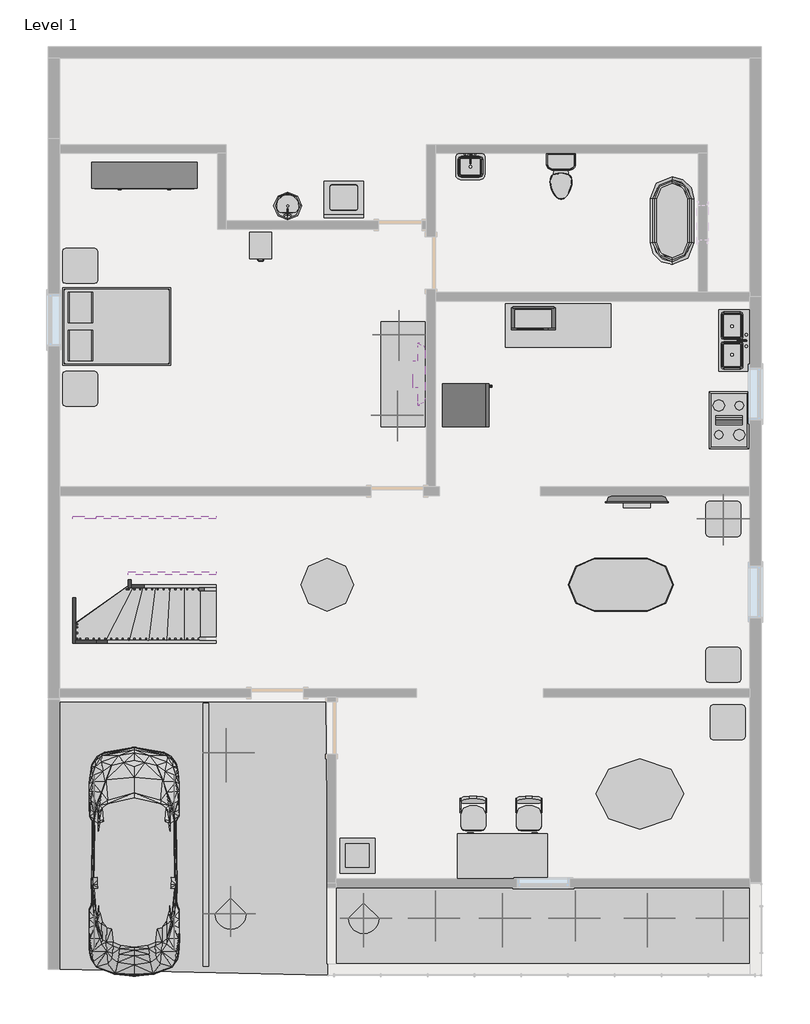
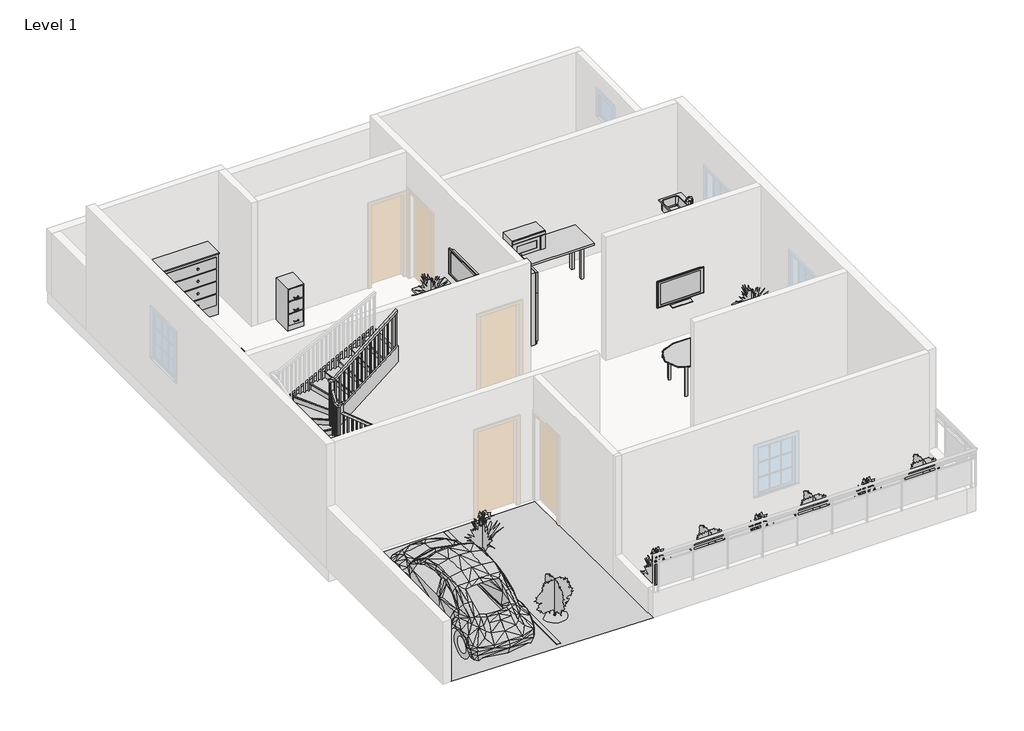
# One storey, part 3 of 3: 19 furniture elements, 11 geographic elements, 8 members, 8 proxies, 7 flow terminals, 1 railing, 1 stair flight.
"""IFC4 building model written with IfcOpenShell, lengths in millimetres."""

from ifc_helpers import new_model, si_unit, frame, origin, place, context, project, spatial, polyline, outline, extrude, faceted_brep, triangles, transform, mapped, element, save
from components import proxy_bb1e6e30, proxy_8a8d5ab2, parking_space_9_x_18_90_deg_85bc4432, rpc_beetle_rpc_beetle_3ce7ba48, proxy_a13a33b2, proxy_718fa39f, flow_terminal_accce45a, flow_terminal_5c41af1d, flow_terminal_a53be723, flow_terminal_d49f872f, flow_terminal_62a433f7, toilet_domestic_3d_toilet_domestic_3d_f7549cf7, toilet_domestic_3d_toilet_domestic_3d_183bbd19, flow_terminal_b374fae2, furniture_c8abb964, furniture_552c1472, furniture_013ab306, furniture_7c473f12, furniture_3d1d9cbc, furniture_7a3aaa4f, furniture_b5c51a22, furniture_2c34a4f9, furniture_905aceb5, furniture_743965d2, furniture_5d68651d, furniture_046c8a23, rpc_plant_tropical_55f6ff97, rpc_plant_tropical_agave_1_5_93a2a214, rpc_plant_tropical_jungle_flame_3_9c4808c2, stair_flight_f6e367ce

model = new_model("IFC4")

# Units and contexts
model_context = context("Model", 3, world=origin())
ifc_project = project(units=[si_unit("LENGTHUNIT", "METRE", prefix="MILLI")], contexts=[model_context])

# Site, building, storey
site = spatial("IfcSite", under=ifc_project)
building = spatial("IfcBuilding", under=site)
storey = spatial("IfcBuildingStorey", under=building, Name="Level 1", Elevation=0.0)

# Proxies
placement = place(None, origin())
element("IfcBuildingElementProxy", 1, Name="Building Element Proxy", at=placement, inside=storey, context=model_context, shape_type="Tessellation", body=[
    triangles([(-12521.6229034, 814.3117052, 0.0), (-7898.8236786, 776.2117052, 0.0), (-7860.7236786, -3973.5882706, 0.0), (-12521.6229034, -3871.9883675, 0.0), (-7898.8236786, 852.4117052, 0.0), (-12521.6229034, 839.711681, 0.0)], [[2, 5, 1], [1, 4, 2], [6, 1, 5], [2, 3, 5], [3, 2, 4]], closed=False),
])
element("IfcBuildingElementProxy", 2, Name="Building Element Proxy", at=placement, inside=storey, context=model_context, shape_type="Tessellation", body=[
    triangles([(-7873.4234848, -2449.5882706, 0.0), (-7860.7236786, -3770.3881737, 0.0), (-532.8234727, -2449.5882706, 0.0), (-532.8234727, -3770.3881737, 0.0)], [[1, 2, 3], [4, 3, 2]], closed=False),
])
proxy_shape = proxy_bb1e6e30(model_context)
element("IfcBuildingElementProxy", 3, Name="Cook Top-4 Unit : 36\" x 20\"", ObjectType="Cook Top-4 Unit : 36\" x 20\"", at=placement, inside=storey, context=model_context, shape_type="MappedRepresentation", body=[
    mapped(proxy_shape, transform((-888.4234692, 5665.7116886, 0.0), x_axis=(0.0, -1.0000000000000004, 0.0), y_axis=(1.0000000000000004, 0.0, 0.0), z_axis=(0.0, 0.0, 1.0))),
])
proxy_2_shape = proxy_8a8d5ab2(model_context)
element("IfcBuildingElementProxy", 4, Name="Microwave : 30\" x 16\" x 18\"", ObjectType="Microwave : 30\" x 16\" x 18\"", at=placement, inside=storey, context=model_context, shape_type="MappedRepresentation", body=[
    mapped(proxy_2_shape, transform((-4792.3163465, 7790.4421944, 0.0), x_axis=(1.0, 0.0, 0.0), y_axis=(0.0, 1.0, 0.0), z_axis=(0.0, 0.0, 1.0))),
])
parking_space_9_x_18_90_deg_shape = parking_space_9_x_18_90_deg_85bc4432(model_context)
element("IfcBuildingElementProxy", 5, Name="Parking Space : 9' x 18' - 90 deg", ObjectType="Parking Space : 9' x 18' - 90 deg", at=placement, inside=storey, context=model_context, shape_type="MappedRepresentation", body=[
    mapped(parking_space_9_x_18_90_deg_shape, transform((-9981.6234692, -3821.1883114, 0.0), x_axis=(-1.0, 0.0, 0.0), y_axis=(0.0, -1.0, 0.0), z_axis=(0.0, 0.0, 1.0))),
])
rpc_beetle_rpc_beetle_shape = rpc_beetle_rpc_beetle_3ce7ba48(model_context)
element("IfcBuildingElementProxy", 6, Name="RPC Beetle : RPC Beetle", ObjectType="RPC Beetle : RPC Beetle", at=placement, inside=storey, context=model_context, shape_type="MappedRepresentation", body=[
    mapped(rpc_beetle_rpc_beetle_shape, transform((-11226.2234692, -3236.9883114, 0.0), x_axis=(1.0, 0.0, 0.0), y_axis=(0.0, 1.0, 0.0), z_axis=(0.0, 0.0, 1.0))),
])
proxy_3_shape = proxy_a13a33b2(model_context)
element("IfcBuildingElementProxy", 7, Name="Refrigerator : 30\" x 32\" RH", ObjectType="Refrigerator : 30\" x 32\" RH", at=placement, inside=storey, context=model_context, shape_type="MappedRepresentation", body=[
    mapped(proxy_3_shape, transform((-5477.8859692, 5924.8627171, 0.0), x_axis=(0.0, 1.0000000000000002, 0.0), y_axis=(-1.0000000000000002, 0.0, 0.0), z_axis=(0.0, 0.0, 1.0))),
])
proxy_4_shape = proxy_718fa39f(model_context)
element("IfcBuildingElementProxy", 8, Name="Washer : 27\" x 25\" x 35\"", ObjectType="Washer : 27\" x 25\" x 35\"", at=placement, inside=storey, context=model_context, shape_type="MappedRepresentation", body=[
    mapped(proxy_4_shape, transform((-7163.5409376, 9780.7621238, 0.0), x_axis=(-1.0000000000000004, 0.0, 0.0), y_axis=(0.0, -1.0000000000000004, 0.0), z_axis=(0.0, 0.0, 1.0))),
])

# Flow terminals
flow_terminal_shape = flow_terminal_accce45a(model_context)
element("IfcFlowTerminal", 9, ObjectType="Floor Drain - Round : 5\" Strainer - 2\" Drain", at=placement, inside=storey, context=model_context, shape_type="MappedRepresentation", body=[
    mapped(flow_terminal_shape, transform((-2666.4234692, 9818.6116886, 0.0), x_axis=(1.0, 0.0, 0.0), y_axis=(0.0, 1.0, 0.0), z_axis=(0.0, 0.0, 1.0))),
])
flow_terminal_2_shape = flow_terminal_5c41af1d(model_context)
element("IfcFlowTerminal", 10, ObjectType="Floor Drain - Round : 5\" Strainer - 4\" Drain", at=placement, inside=storey, context=model_context, shape_type="MappedRepresentation", body=[
    mapped(flow_terminal_2_shape, transform((-8406.8234692, 9386.8116886, 0.0), x_axis=(1.0, 0.0, 0.0), y_axis=(0.0, 1.0, 0.0), z_axis=(0.0, 0.0, 1.0))),
])
flow_terminal_3_shape = flow_terminal_a53be723(model_context)
element("IfcFlowTerminal", 11, ObjectType="Sink Kitchen-Double : 42\" x 21\"", at=placement, inside=storey, context=model_context, shape_type="MappedRepresentation", body=[
    mapped(flow_terminal_3_shape, transform((-801.8201514, 7065.7009292, 0.0), x_axis=(0.0, -1.0000000000000002, 0.0), y_axis=(1.0000000000000002, 0.0, 0.0), z_axis=(0.0, 0.0, 1.0))),
])
flow_terminal_4_shape = flow_terminal_d49f872f(model_context)
element("IfcFlowTerminal", 12, ObjectType="Sink Vanity-Round : 19\" x 19\"", at=placement, inside=storey, context=model_context, shape_type="MappedRepresentation", body=[
    mapped(flow_terminal_4_shape, transform((-8462.5717286, 9471.7478463, 0.0), x_axis=(-1.0000000000000004, 0.0, 0.0), y_axis=(0.0, -1.0000000000000004, 0.0), z_axis=(0.0, 0.0, 1.0))),
])
flow_terminal_5_shape = flow_terminal_62a433f7(model_context)
element("IfcFlowTerminal", 13, ObjectType="Sink Vanity-Square : 20\" x 18\"", at=placement, inside=storey, context=model_context, shape_type="MappedRepresentation", body=[
    mapped(flow_terminal_5_shape, transform((-5399.9127097, 10121.0662875, 0.0), x_axis=(1.0, 0.0, 0.0), y_axis=(0.0, 1.0, 0.0), z_axis=(0.0, 0.0, 1.0))),
])
toilet_domestic_3d_toilet_domestic_3d_shape = toilet_domestic_3d_toilet_domestic_3d_f7549cf7(model_context)
toilet_domestic_3d_toilet_domestic_3d_2_shape = toilet_domestic_3d_toilet_domestic_3d_183bbd19(model_context)
element("IfcFlowTerminal", 14, ObjectType="Toilet-Domestic-3D : Toilet-Domestic-3D", at=placement, inside=storey, context=model_context, shape_type="MappedRepresentation", body=[
    mapped(toilet_domestic_3d_toilet_domestic_3d_shape, transform((-3809.4234692, 9806.5156613, 0.0), x_axis=(1.0, 0.0, 0.0), y_axis=(0.0, 1.0, 0.0), z_axis=(0.0, 0.0, 1.0))),
    mapped(toilet_domestic_3d_toilet_domestic_3d_2_shape, transform((-3809.4234692, 9806.5156613, 0.0), x_axis=(1.0, 0.0, 0.0), y_axis=(0.0, 1.0, 0.0), z_axis=(0.0, 0.0, 1.0))),
])
flow_terminal_6_shape = flow_terminal_b374fae2(model_context)
element("IfcFlowTerminal", 15, ObjectType="Tub-Free Standing-3D : 30\" x 60\"", at=placement, inside=storey, context=model_context, shape_type="MappedRepresentation", body=[
    mapped(flow_terminal_6_shape, transform((-1879.0234692, 9132.8116886, 0.0), x_axis=(1.0, 0.0, 0.0), y_axis=(0.0, 1.0, 0.0), z_axis=(0.0, 0.0, 1.0))),
])

# Furniture
furniture_shape = furniture_c8abb964(model_context)
element("IfcFurniture", 16, ObjectType="Bed-Box : Double 53\" x 74\"", at=placement, inside=storey, context=model_context, shape_type="MappedRepresentation", body=[
    mapped(furniture_shape, transform((-11765.4529773, 6952.1592296, 0.0), x_axis=(0.0, 1.0, 0.0), y_axis=(-1.0, 0.0, 0.0), z_axis=(0.0, 0.0, 1.0))),
])
furniture_2_shape = furniture_552c1472(model_context)
element("IfcFurniture", 17, ObjectType="Cabinet-File 3 Drawer : 15\" x 18\"", at=placement, inside=storey, context=model_context, shape_type="MappedRepresentation", body=[
    mapped(furniture_2_shape, transform((-8901.2270221, 8843.1459887, 0.0), x_axis=(1.0, 0.0, 0.0), y_axis=(0.0, 1.0, 0.0), z_axis=(0.0, 0.0, 1.0))),
])
furniture_3_shape = furniture_013ab306(model_context)
element("IfcFurniture", 18, ObjectType="Desk : 60\" x 30\" Student", at=placement, inside=storey, context=model_context, shape_type="MappedRepresentation", body=[
    mapped(furniture_3_shape, transform((-4063.4234692, -1535.1883114, 0.0), x_axis=(-1.0000000000000004, 0.0, 0.0), y_axis=(0.0, -1.0000000000000004, 0.0), z_axis=(0.0, 0.0, 1.0))),
])
furniture_4_shape = furniture_7c473f12(model_context)
element("IfcFurniture", 19, ObjectType="Dresser : 72\" x 60\" x 18\"", at=placement, inside=storey, context=model_context, shape_type="MappedRepresentation", body=[
    mapped(furniture_4_shape, transform((-10779.2302093, 10283.3746427, 0.0), x_axis=(1.0000000000000009, 0.0, 0.0), y_axis=(0.0, 1.0000000000000009, 0.0), z_axis=(0.0, 0.0, 1.0))),
])
furniture_5_shape = furniture_3d1d9cbc(model_context)
element("IfcFurniture", 20, ObjectType="Seating-Auditorium : 18\" x 24\" x 30\"", at=placement, inside=storey, context=model_context, shape_type="MappedRepresentation", body=[
    mapped(furniture_5_shape, transform((-5172.6956003, -964.3129015, 0.0), x_axis=(-1.0000000000000004, 0.0, 0.0), y_axis=(0.0, -1.0000000000000004, 0.0), z_axis=(0.0, 0.0, 1.0))),
])
element("IfcFurniture", 21, ObjectType="Seating-Auditorium : 18\" x 24\" x 30\"", at=placement, inside=storey, context=model_context, shape_type="MappedRepresentation", body=[
    mapped(furniture_5_shape, transform((-4207.4956003, -964.3129015, 0.0), x_axis=(-1.0000000000000004, 0.0, 0.0), y_axis=(0.0, -1.0000000000000004, 0.0), z_axis=(0.0, 0.0, 1.0))),
])
furniture_6_shape = furniture_7a3aaa4f(model_context)
element("IfcFurniture", 22, ObjectType="TV - Flat Screen : 42\"", at=placement, inside=storey, context=model_context, shape_type="MappedRepresentation", body=[
    mapped(furniture_6_shape, transform((-6227.9045549, 6461.8671745, 1219.2), x_axis=(0.0, -1.0000000000000004, 0.0), y_axis=(1.0000000000000004, 0.0, 0.0), z_axis=(0.0, 0.0, 1.0))),
])
element("IfcFurniture", 23, ObjectType="TV - Flat Screen : 42\"", at=placement, inside=storey, context=model_context, shape_type="MappedRepresentation", body=[
    mapped(furniture_6_shape, transform((-2484.678955, 4299.073065, 914.4), x_axis=(1.0, 0.0, 0.0), y_axis=(0.0, 1.0, 0.0), z_axis=(0.0, 0.0, 1.0))),
])
furniture_7_shape = furniture_b5c51a22(model_context)
element("IfcFurniture", 24, ObjectType="Table-Coffee : 24\" x 24\" x 24\"", at=placement, inside=storey, context=model_context, shape_type="MappedRepresentation", body=[
    mapped(furniture_7_shape, transform((-7364.6392358, -1992.3493892, 0.0), x_axis=(1.0, 0.0, 0.0), y_axis=(0.0, 1.0, 0.0), z_axis=(0.0, 0.0, 1.0))),
])
furniture_8_shape = furniture_2c34a4f9(model_context)
element("IfcFurniture", 25, ObjectType="Table-Dining Oval : 36\" x 72\"", at=placement, inside=storey, context=model_context, shape_type="MappedRepresentation", body=[
    mapped(furniture_8_shape, transform((-3169.8431413, 2450.113328, 0.0), x_axis=(-1.0000000000000004, 0.0, 0.0), y_axis=(0.0, -1.0000000000000004, 0.0), z_axis=(0.0, 0.0, 1.0))),
])
furniture_9_shape = furniture_905aceb5(model_context)
element("IfcFurniture", 26, ObjectType="Table-Dining Round w Chairs : 36\" Diameter", at=placement, inside=storey, context=model_context, shape_type="MappedRepresentation", body=[
    mapped(furniture_9_shape, transform((-7977.1054364, 2993.0903771, 0.0), x_axis=(1.0, 0.0, 0.0), y_axis=(0.0, 1.0, 0.0), z_axis=(0.0, 0.0, 1.0))),
])
furniture_10_shape = furniture_743965d2(model_context)
element("IfcFurniture", 27, ObjectType="Table-Ellipse : 60\" x 48\"", at=placement, inside=storey, context=model_context, shape_type="MappedRepresentation", body=[
    mapped(furniture_10_shape, transform((-2437.8234692, -823.9883114, 0.0), x_axis=(1.0, 0.0, 0.0), y_axis=(0.0, 1.0, 0.0), z_axis=(0.0, 0.0, 1.0))),
])
furniture_11_shape = furniture_5d68651d(model_context)
element("IfcFurniture", 28, ObjectType="Table-End : 24\" x 24\"", at=placement, inside=storey, context=model_context, shape_type="MappedRepresentation", body=[
    mapped(furniture_11_shape, transform((-12474.5570994, 6059.4116886, 0.0), x_axis=(1.0, 0.0, 0.0), y_axis=(0.0, 1.0, 0.0), z_axis=(0.0, 0.0, 1.0))),
])
element("IfcFurniture", 29, ObjectType="Table-End : 24\" x 24\"", at=placement, inside=storey, context=model_context, shape_type="MappedRepresentation", body=[
    mapped(furniture_11_shape, transform((-12474.5570994, 8193.0116886, 0.0), x_axis=(1.0, 0.0, 0.0), y_axis=(0.0, 1.0, 0.0), z_axis=(0.0, 0.0, 1.0))),
])
element("IfcFurniture", 30, ObjectType="Table-End : 24\" x 24\"", at=placement, inside=storey, context=model_context, shape_type="MappedRepresentation", body=[
    mapped(furniture_11_shape, transform((-1298.5570994, 3798.8116886, 0.0), x_axis=(1.0, 0.0, 0.0), y_axis=(0.0, 1.0, 0.0), z_axis=(0.0, 0.0, 1.0))),
])
element("IfcFurniture", 31, ObjectType="Table-End : 24\" x 24\"", at=placement, inside=storey, context=model_context, shape_type="MappedRepresentation", body=[
    mapped(furniture_11_shape, transform((-1298.5570994, 1265.1616886, 0.0), x_axis=(1.0, 0.0, 0.0), y_axis=(0.0, 1.0, 0.0), z_axis=(0.0, 0.0, 1.0))),
])
element("IfcFurniture", 32, ObjectType="Table-End : 24\" x 24\"", at=placement, inside=storey, context=model_context, shape_type="MappedRepresentation", body=[
    mapped(furniture_11_shape, transform((-1222.3570994, 268.2116886, 0.0), x_axis=(1.0, 0.0, 0.0), y_axis=(0.0, 1.0, 0.0), z_axis=(0.0, 0.0, 1.0))),
])
furniture_12_shape = furniture_046c8a23(model_context)
element("IfcFurniture", 33, ObjectType="Table-Rectangular : 72\" x 30\"", at=placement, inside=storey, context=model_context, shape_type="MappedRepresentation", body=[
    mapped(furniture_12_shape, transform((-6552.6234692, 6465.8116886, 0.0), x_axis=(0.0, 1.0000000000000002, 0.0), y_axis=(-1.0000000000000002, 0.0, 0.0), z_axis=(0.0, 0.0, 1.0))),
])
element("IfcFurniture", 34, ObjectType="Table-Rectangular : 72\" x 30\"", at=placement, inside=storey, context=model_context, shape_type="MappedRepresentation", body=[
    mapped(furniture_12_shape, transform((-3860.2234692, 7310.3616886, 0.0), x_axis=(1.0, 0.0, 0.0), y_axis=(0.0, 1.0, 0.0), z_axis=(0.0, 0.0, 1.0))),
])

# Geographic elements
rpc_plant_tropical_shape = rpc_plant_tropical_55f6ff97(model_context)
element("IfcGeographicElement", 35, ObjectType="RPC Plant - Tropical", at=placement, inside=storey, context=model_context, shape_type="MappedRepresentation", body=[
    mapped(rpc_plant_tropical_shape, transform((-7238.4234692, -2982.9883114, 0.0), x_axis=(1.0, 0.0, 0.0), y_axis=(0.0, 1.0, 0.0), z_axis=(0.0, 0.0, 1.0))),
])
element("IfcGeographicElement", 36, ObjectType="RPC Plant - Tropical", at=placement, inside=storey, context=model_context, shape_type="MappedRepresentation", body=[
    mapped(rpc_plant_tropical_shape, transform((-2310.8234692, -2982.9883114, 0.0), x_axis=(1.0, 0.0, 0.0), y_axis=(0.0, 1.0, 0.0), z_axis=(0.0, 0.0, 1.0))),
])
element("IfcGeographicElement", 37, ObjectType="RPC Plant - Tropical", at=placement, inside=storey, context=model_context, shape_type="MappedRepresentation", body=[
    mapped(rpc_plant_tropical_shape, transform((-4825.4234692, -2982.9883114, 0.0), x_axis=(1.0, 0.0, 0.0), y_axis=(0.0, 1.0, 0.0), z_axis=(0.0, 0.0, 1.0))),
])
element("IfcGeographicElement", 38, ObjectType="RPC Plant - Tropical", at=placement, inside=storey, context=model_context, shape_type="MappedRepresentation", body=[
    mapped(rpc_plant_tropical_shape, transform((-9626.0234692, -112.7883114, 0.0), x_axis=(1.0, 0.0, 0.0), y_axis=(0.0, 1.0, 0.0), z_axis=(0.0, 0.0, 1.0))),
])
rpc_plant_tropical_agave_1_5_shape = rpc_plant_tropical_agave_1_5_93a2a214(model_context)
element("IfcGeographicElement", 39, ObjectType="RPC Plant - Tropical : Agave - 1.5'", at=placement, inside=storey, context=model_context, shape_type="MappedRepresentation", body=[
    mapped(rpc_plant_tropical_agave_1_5_shape, transform((-6628.8234692, 7151.6116886, 762.0), x_axis=(1.0, 0.0, 0.0), y_axis=(0.0, 1.0, 0.0), z_axis=(0.0, 0.0, 1.0))),
])
element("IfcGeographicElement", 40, ObjectType="RPC Plant - Tropical : Agave - 1.5'", at=placement, inside=storey, context=model_context, shape_type="MappedRepresentation", body=[
    mapped(rpc_plant_tropical_agave_1_5_shape, transform((-6654.2234692, 5754.6116886, 762.0), x_axis=(1.0, 0.0, 0.0), y_axis=(0.0, 1.0, 0.0), z_axis=(0.0, 0.0, 1.0))),
])
element("IfcGeographicElement", 41, ObjectType="RPC Plant - Tropical : Agave - 1.5'", at=placement, inside=storey, context=model_context, shape_type="MappedRepresentation", body=[
    mapped(rpc_plant_tropical_agave_1_5_shape, transform((-990.0234692, 3951.2116886, 457.2), x_axis=(1.0, 0.0, 0.0), y_axis=(0.0, 1.0, 0.0), z_axis=(0.0, 0.0, 1.0))),
])
rpc_plant_tropical_jungle_flame_3_shape = rpc_plant_tropical_jungle_flame_3_9c4808c2(model_context)
element("IfcGeographicElement", 42, ObjectType="RPC Plant - Tropical : Jungle Flame - 3'", at=placement, inside=storey, context=model_context, shape_type="MappedRepresentation", body=[
    mapped(rpc_plant_tropical_jungle_flame_3_shape, transform((-990.0234692, -2982.9883114, 0.0), x_axis=(1.0, 0.0, 0.0), y_axis=(0.0, 1.0, 0.0), z_axis=(0.0, 0.0, 1.0))),
])
element("IfcGeographicElement", 43, ObjectType="RPC Plant - Tropical : Jungle Flame - 3'", at=placement, inside=storey, context=model_context, shape_type="MappedRepresentation", body=[
    mapped(rpc_plant_tropical_jungle_flame_3_shape, transform((-3555.4234692, -2982.9883114, 0.0), x_axis=(1.0, 0.0, 0.0), y_axis=(0.0, 1.0, 0.0), z_axis=(0.0, 0.0, 1.0))),
])
element("IfcGeographicElement", 44, ObjectType="RPC Plant - Tropical : Jungle Flame - 3'", at=placement, inside=storey, context=model_context, shape_type="MappedRepresentation", body=[
    mapped(rpc_plant_tropical_jungle_flame_3_shape, transform((-5993.8234692, -2982.9883114, 0.0), x_axis=(1.0, 0.0, 0.0), y_axis=(0.0, 1.0, 0.0), z_axis=(0.0, 0.0, 1.0))),
])
element("IfcGeographicElement", 45, ObjectType="RPC Plant - Tropical : Jungle Flame - 3'", at=placement, inside=storey, context=model_context, shape_type="MappedRepresentation", body=[
    mapped(rpc_plant_tropical_jungle_flame_3_shape, transform((-9549.8234692, -2906.7883114, 0.0), x_axis=(1.0, 0.0, 0.0), y_axis=(0.0, 1.0, 0.0), z_axis=(0.0, 0.0, 1.0))),
])

# Members
element("IfcMember", 46, ObjectType="Stringer - 2\" Width", at=placement, inside=storey, context=model_context, shape_type="SweptSolid", body=[
    extrude(outline(polyline([(0.0, -9800.0917773), (229.639954, -9800.0917773), (1305.3956453, -11887.508969), (962.500629, -11887.508969), (0.0, -10019.8540949), (0.0, -9800.0917773)])), frame((0.0, 1792.2116886, 0.0), z_axis=(0.0, 1.0, 0.0), x_axis=(0.0, 0.0, 1.0)), (0.0, 0.0, 1.0), 50.8),
])
element("IfcMember", 47, ObjectType="Stringer - 2\" Width", at=placement, inside=storey, context=model_context, shape_type="SweptSolid", body=[
    extrude(outline(polyline([(-11887.508969, 1843.0116886), (-11887.508969, 1792.2116886), (-12242.2234692, 1792.2116886), (-12242.2234692, 1843.0116886), (-11887.508969, 1843.0116886)])), frame((0.0, 0.0, 962.500629), z_axis=(0.0, 0.0, 1.0), x_axis=(1.0, 0.0, 0.0)), (0.0, 0.0, 1.0), 342.8950162),
])
element("IfcMember", 48, ObjectType="Stringer - 2\" Width", at=placement, inside=storey, context=model_context, shape_type="SweptSolid", body=[
    extrude(outline(polyline([(1792.2116886, 1000.5956453), (1792.2116886, 1289.0952212), (3914.2315713, 1969.9972697), (3951.2116886, 1969.9972697), (3951.2116886, 1638.9682298), (1961.7341716, 1000.5956453), (1792.2116886, 1000.5956453)])), frame((-12293.0234692, 0.0, 0.0), z_axis=(1.0, 0.0, 0.0), x_axis=(0.0, 1.0, 0.0)), (0.0, 0.0, 1.0), 50.8),
])
element("IfcMember", 49, ObjectType="Stringer - 2\" Width", at=placement, inside=storey, context=model_context, shape_type="SweptSolid", body=[
    extrude(outline(polyline([(-12293.0234692, 3951.2116886), (-12293.0234692, 4002.0116886), (-11887.508969, 4002.0116886), (-11887.508969, 3951.2116886), (-12293.0234692, 3951.2116886)])), frame((0.0, 0.0, 1649.8904473), z_axis=(0.0, 0.0, 1.0), x_axis=(1.0, 0.0, 0.0)), (0.0, 0.0, 1.0), 320.1068224),
])
element("IfcMember", 50, ObjectType="Stringer - 2\" Width", at=placement, inside=storey, context=model_context, shape_type="SweptSolid", body=[
    extrude(outline(polyline([(1969.9972697, -11887.508969), (1649.8904473, -11887.508969), (2725.6461385, -9800.0917773), (3045.7529609, -9800.0917773), (1969.9972697, -11887.508969)])), frame((0.0, 3951.2116886, 0.0), z_axis=(0.0, 1.0, 0.0), x_axis=(0.0, 0.0, 1.0)), (0.0, 0.0, 1.0), 50.8),
])
element("IfcMember", 51, ObjectType="Stringer - 2\" Width", at=placement, inside=storey, context=model_context, shape_type="SweptSolid", body=[
    extrude(outline(polyline([(0.0, -9800.0917773), (176.1764461, -9800.0917773), (1380.418648, -11277.0234692), (987.1410923, -11277.0234692), (0.0, -10066.3534218), (0.0, -9800.0917773)])), frame((0.0, 2757.4116886, 0.0), z_axis=(0.0, 1.0, 0.0), x_axis=(0.0, 0.0, 1.0)), (0.0, 0.0, 1.0), 50.8),
])
element("IfcMember", 52, ObjectType="Stringer - 2\" Width", at=placement, inside=storey, context=model_context, shape_type="SweptSolid", body=[
    extrude(outline(polyline([(2757.4116886, 1028.5617647), (2757.4116886, 1573.2682978), (2964.048806, 1926.1409689), (2986.0116886, 1926.1409689), (2986.0116886, 1360.465107), (2791.6539059, 1028.5617647), (2757.4116886, 1028.5617647)])), frame((-11327.8234692, 0.0, 0.0), z_axis=(1.0, 0.0, 0.0), x_axis=(0.0, 1.0, 0.0)), (0.0, 0.0, 1.0), 50.8),
])
element("IfcMember", 53, ObjectType="Stringer - 2\" Width", at=placement, inside=storey, context=model_context, shape_type="SweptSolid", body=[
    extrude(outline(polyline([(1926.1409689, -11327.8234692), (1532.8634131, -11327.8234692), (2778.5262875, -9800.0917773), (3171.8038432, -9800.0917773), (1926.1409689, -11327.8234692)])), frame((0.0, 2986.0116886, 0.0), z_axis=(0.0, 1.0, 0.0), x_axis=(0.0, 0.0, 1.0)), (0.0, 0.0, 1.0), 50.8),
])

# Railing
element("IfcRailing", 54, ObjectType="Handrail - Rectangular", at=placement, inside=storey, context=model_context, shape_type="SolidModel", body=[
    faceted_brep([(-9800.0917773, 2706.6116886, 1025.2529681), (-9800.0917773, 2706.6116886, 959.7067088), (-9800.0917773, 2757.4116886, 959.7067088), (-9800.0917773, 2757.4116886, 1025.2529681), (-11251.6234692, 2706.6116886, 2208.7848338), (-11302.4234692, 2706.6116886, 2184.659247), (-11302.4234692, 2757.4116886, 2184.659247), (-11251.6234692, 2757.4116886, 2208.7848338), (-11251.6234692, 2706.6116886, 2414.6281882), (-11302.4234692, 2706.6116886, 2363.8281882), (-11302.4234692, 2757.4116886, 2363.8281882), (-11251.6234692, 2757.4116886, 2414.6281882), (-11378.6234692, 2706.6116886, 2414.6281882), (-11378.6234692, 2706.6116886, 2363.8281882), (-11327.8234692, 2757.4116886, 2363.8281882), (-11327.8234692, 2757.4116886, 2414.6281882), (-11378.6234692, 2833.6116886, 2414.6281882), (-11378.6234692, 2862.7330225, 2363.8281882), (-11327.8234692, 2862.7330225, 2363.8281882), (-11327.8234692, 2833.6116886, 2414.6281882), (-11378.6234692, 2960.6116886, 2631.5051451), (-11378.6234692, 3011.4116886, 2617.7256424), (-11327.8234692, 3011.4116886, 2617.7256424), (-11327.8234692, 2960.6116886, 2631.5051451), (-11378.6234692, 2960.6116886, 2837.3484995), (-11378.6234692, 3011.4116886, 2786.5484995), (-11327.8234692, 3011.4116886, 2786.5484995), (-11327.8234692, 2960.6116886, 2837.3484995), (-11378.6234692, 3087.6116886, 2837.3484995), (-11378.6234692, 3087.6116886, 2786.5484995), (-11327.8234692, 3036.8116886, 2786.5484995), (-11327.8234692, 3036.8116886, 2837.3484995), (-11251.6234692, 3087.6116886, 2837.3484995), (-11233.5380561, 3087.6116886, 2786.5484995), (-11233.5380561, 3036.8116886, 2786.5484995), (-11251.6234692, 3036.8116886, 2837.3484995), (-9800.0917773, 3087.6116886, 4020.8803652), (-9800.0917773, 3036.8116886, 4020.8803652), (-9800.0917773, 3036.8116886, 3955.3341059), (-9800.0917773, 3087.6116886, 3955.3341059)], [[[0, 1, 2, 3]], [[1, 0, 4, 5]], [[2, 1, 5, 6]], [[3, 2, 6, 7]], [[0, 3, 7, 4]], [[5, 4, 8, 9]], [[6, 5, 9, 10]], [[7, 6, 10, 11]], [[4, 7, 11, 8]], [[9, 8, 12, 13]], [[10, 9, 13, 14]], [[11, 10, 14, 15]], [[8, 11, 15, 12]], [[13, 12, 16, 17]], [[14, 13, 17, 18]], [[15, 14, 18, 19]], [[12, 15, 19, 16]], [[17, 16, 20, 21]], [[18, 17, 21, 22]], [[19, 18, 22, 23]], [[16, 19, 23, 20]], [[21, 20, 24, 25]], [[22, 21, 25, 26]], [[23, 22, 26, 27]], [[20, 23, 27, 24]], [[25, 24, 28, 29]], [[26, 25, 29, 30]], [[27, 26, 30, 31]], [[24, 27, 31, 28]], [[29, 28, 32, 33]], [[30, 29, 33, 34]], [[31, 30, 34, 35]], [[28, 31, 35, 32]], [[36, 37, 38, 39]], [[33, 32, 36, 39]], [[34, 33, 39, 38]], [[35, 34, 38, 37]], [[32, 35, 37, 36]]]),
    extrude(outline(polyline([(3881.7558784, -9890.3311128), (3866.2231262, -9909.3811128), (2878.6666667, -9909.3811128), (2878.6666667, -9890.3311128), (3881.7558784, -9890.3311128)])), frame((0.0, 3052.6866886, 0.0), z_axis=(0.0, 1.0, 0.0), x_axis=(0.0, 0.0, 1.0)), (0.0, 0.0, 1.0), 19.05),
    extrude(outline(polyline([(3798.9145334, -9991.9311128), (3783.3817813, -10010.9811128), (2878.6666667, -10010.9811128), (2878.6666667, -9991.9311128), (3798.9145334, -9991.9311128)])), frame((0.0, 3052.6866886, 0.0), z_axis=(0.0, 1.0, 0.0), x_axis=(0.0, 0.0, 1.0)), (0.0, 0.0, 1.0), 19.05),
    extrude(outline(polyline([(3716.0731885, -10093.5311128), (3700.5404364, -10112.5811128), (2709.3333333, -10112.5811128), (2709.3333333, -10093.5311128), (3716.0731885, -10093.5311128)])), frame((0.0, 3052.6866886, 0.0), z_axis=(0.0, 1.0, 0.0), x_axis=(0.0, 0.0, 1.0)), (0.0, 0.0, 1.0), 19.05),
    extrude(outline(polyline([(3633.2318436, -10195.1311128), (3617.6990914, -10214.1811128), (2709.3333333, -10214.1811128), (2709.3333333, -10195.1311128), (3633.2318436, -10195.1311128)])), frame((0.0, 3052.6866886, 0.0), z_axis=(0.0, 1.0, 0.0), x_axis=(0.0, 0.0, 1.0)), (0.0, 0.0, 1.0), 19.05),
    extrude(outline(polyline([(3550.3904987, -10296.7311128), (3534.8577465, -10315.7811128), (2709.3333333, -10315.7811128), (2709.3333333, -10296.7311128), (3550.3904987, -10296.7311128)])), frame((0.0, 3052.6866886, 0.0), z_axis=(0.0, 1.0, 0.0), x_axis=(0.0, 0.0, 1.0)), (0.0, 0.0, 1.0), 19.05),
    extrude(outline(polyline([(3467.5491538, -10398.3311128), (3452.0164016, -10417.3811128), (2540.0, -10417.3811128), (2540.0, -10398.3311128), (3467.5491538, -10398.3311128)])), frame((0.0, 3052.6866886, 0.0), z_axis=(0.0, 1.0, 0.0), x_axis=(0.0, 0.0, 1.0)), (0.0, 0.0, 1.0), 19.05),
    extrude(outline(polyline([(3384.7078088, -10499.9311128), (3369.1750567, -10518.9811128), (2540.0, -10518.9811128), (2540.0, -10499.9311128), (3384.7078088, -10499.9311128)])), frame((0.0, 3052.6866886, 0.0), z_axis=(0.0, 1.0, 0.0), x_axis=(0.0, 0.0, 1.0)), (0.0, 0.0, 1.0), 19.05),
    extrude(outline(polyline([(3301.8664639, -10601.5311128), (3286.3337117, -10620.5811128), (2540.0, -10620.5811128), (2540.0, -10601.5311128), (3301.8664639, -10601.5311128)])), frame((0.0, 3052.6866886, 0.0), z_axis=(0.0, 1.0, 0.0), x_axis=(0.0, 0.0, 1.0)), (0.0, 0.0, 1.0), 19.05),
    extrude(outline(polyline([(3219.025119, -10703.1311128), (3203.4923668, -10722.1811128), (2370.6666667, -10722.1811128), (2370.6666667, -10703.1311128), (3219.025119, -10703.1311128)])), frame((0.0, 3052.6866886, 0.0), z_axis=(0.0, 1.0, 0.0), x_axis=(0.0, 0.0, 1.0)), (0.0, 0.0, 1.0), 19.05),
    extrude(outline(polyline([(3136.1837741, -10804.7311128), (3120.6510219, -10823.7811128), (2370.6666667, -10823.7811128), (2370.6666667, -10804.7311128), (3136.1837741, -10804.7311128)])), frame((0.0, 3052.6866886, 0.0), z_axis=(0.0, 1.0, 0.0), x_axis=(0.0, 0.0, 1.0)), (0.0, 0.0, 1.0), 19.05),
    extrude(outline(polyline([(3053.3424291, -10906.3311128), (3037.809677, -10925.3811128), (2201.3333333, -10925.3811128), (2201.3333333, -10906.3311128), (3053.3424291, -10906.3311128)])), frame((0.0, 3052.6866886, 0.0), z_axis=(0.0, 1.0, 0.0), x_axis=(0.0, 0.0, 1.0)), (0.0, 0.0, 1.0), 19.05),
    extrude(outline(polyline([(2970.5010842, -11007.9311128), (2954.9683321, -11026.9811128), (2201.3333333, -11026.9811128), (2201.3333333, -11007.9311128), (2970.5010842, -11007.9311128)])), frame((0.0, 3052.6866886, 0.0), z_axis=(0.0, 1.0, 0.0), x_axis=(0.0, 0.0, 1.0)), (0.0, 0.0, 1.0), 19.05),
    extrude(outline(polyline([(2887.6597393, -11109.5311128), (2872.1269871, -11128.5811128), (2032.0, -11128.5811128), (2032.0, -11109.5311128), (2887.6597393, -11109.5311128)])), frame((0.0, 3052.6866886, 0.0), z_axis=(0.0, 1.0, 0.0), x_axis=(0.0, 0.0, 1.0)), (0.0, 0.0, 1.0), 19.05),
    extrude(outline(polyline([(2804.8183944, -11211.1311128), (2789.2856422, -11230.1811128), (2032.0, -11230.1811128), (2032.0, -11211.1311128), (2804.8183944, -11211.1311128)])), frame((0.0, 3052.6866886, 0.0), z_axis=(0.0, 1.0, 0.0), x_axis=(0.0, 0.0, 1.0)), (0.0, 0.0, 1.0), 19.05),
    extrude(outline(polyline([(2940.4725924, 2496.5834745), (2959.5225924, 2529.115018), (2959.5225924, 1524.0), (2940.4725924, 1524.0), (2940.4725924, 2496.5834745)])), frame((-11362.7484692, 0.0, 0.0), z_axis=(1.0, 0.0, 0.0), x_axis=(0.0, 1.0, 0.0)), (0.0, 0.0, 1.0), 19.05),
    extrude(outline(polyline([(2838.8725924, 2323.0819089), (2857.9225924, 2355.6134525), (2857.9225924, 1524.0), (2838.8725924, 1524.0), (2838.8725924, 2323.0819089)])), frame((-11362.7484692, 0.0, 0.0), z_axis=(1.0, 0.0, 0.0), x_axis=(0.0, 1.0, 0.0)), (0.0, 0.0, 1.0), 19.05),
    extrude(outline(polyline([(2111.7191617, -11212.9667773), (2127.2519138, -11232.0167773), (1016.0, -11232.0167773), (1016.0, -11212.9667773), (2111.7191617, -11212.9667773)])), frame((0.0, 2722.4866886, 0.0), z_axis=(0.0, 1.0, 0.0), x_axis=(0.0, 0.0, 1.0)), (0.0, 0.0, 1.0), 19.05),
    extrude(outline(polyline([(2028.8778167, -11111.3667773), (2044.4105689, -11130.4167773), (1016.0, -11130.4167773), (1016.0, -11111.3667773), (2028.8778167, -11111.3667773)])), frame((0.0, 2722.4866886, 0.0), z_axis=(0.0, 1.0, 0.0), x_axis=(0.0, 0.0, 1.0)), (0.0, 0.0, 1.0), 19.05),
    extrude(outline(polyline([(1946.0364718, -11009.7667773), (1961.569224, -11028.8167773), (846.6666667, -11028.8167773), (846.6666667, -11009.7667773), (1946.0364718, -11009.7667773)])), frame((0.0, 2722.4866886, 0.0), z_axis=(0.0, 1.0, 0.0), x_axis=(0.0, 0.0, 1.0)), (0.0, 0.0, 1.0), 19.05),
    extrude(outline(polyline([(1863.1951269, -10908.1667773), (1878.7278791, -10927.2167773), (846.6666667, -10927.2167773), (846.6666667, -10908.1667773), (1863.1951269, -10908.1667773)])), frame((0.0, 2722.4866886, 0.0), z_axis=(0.0, 1.0, 0.0), x_axis=(0.0, 0.0, 1.0)), (0.0, 0.0, 1.0), 19.05),
    extrude(outline(polyline([(1780.353782, -10806.5667773), (1795.8865341, -10825.6167773), (677.3333333, -10825.6167773), (677.3333333, -10806.5667773), (1780.353782, -10806.5667773)])), frame((0.0, 2722.4866886, 0.0), z_axis=(0.0, 1.0, 0.0), x_axis=(0.0, 0.0, 1.0)), (0.0, 0.0, 1.0), 19.05),
    extrude(outline(polyline([(1697.5124371, -10704.9667773), (1713.0451892, -10724.0167773), (677.3333333, -10724.0167773), (677.3333333, -10704.9667773), (1697.5124371, -10704.9667773)])), frame((0.0, 2722.4866886, 0.0), z_axis=(0.0, 1.0, 0.0), x_axis=(0.0, 0.0, 1.0)), (0.0, 0.0, 1.0), 19.05),
    extrude(outline(polyline([(1614.6710921, -10603.3667773), (1630.2038443, -10622.4167773), (508.0, -10622.4167773), (508.0, -10603.3667773), (1614.6710921, -10603.3667773)])), frame((0.0, 2722.4866886, 0.0), z_axis=(0.0, 1.0, 0.0), x_axis=(0.0, 0.0, 1.0)), (0.0, 0.0, 1.0), 19.05),
    extrude(outline(polyline([(1531.8297472, -10501.7667773), (1547.3624994, -10520.8167773), (508.0, -10520.8167773), (508.0, -10501.7667773), (1531.8297472, -10501.7667773)])), frame((0.0, 2722.4866886, 0.0), z_axis=(0.0, 1.0, 0.0), x_axis=(0.0, 0.0, 1.0)), (0.0, 0.0, 1.0), 19.05),
    extrude(outline(polyline([(1448.9884023, -10400.1667773), (1464.5211545, -10419.2167773), (508.0, -10419.2167773), (508.0, -10400.1667773), (1448.9884023, -10400.1667773)])), frame((0.0, 2722.4866886, 0.0), z_axis=(0.0, 1.0, 0.0), x_axis=(0.0, 0.0, 1.0)), (0.0, 0.0, 1.0), 19.05),
    extrude(outline(polyline([(1366.1470574, -10298.5667773), (1381.6798095, -10317.6167773), (338.6666667, -10317.6167773), (338.6666667, -10298.5667773), (1366.1470574, -10298.5667773)])), frame((0.0, 2722.4866886, 0.0), z_axis=(0.0, 1.0, 0.0), x_axis=(0.0, 0.0, 1.0)), (0.0, 0.0, 1.0), 19.05),
    extrude(outline(polyline([(1283.3057124, -10196.9667773), (1298.8384646, -10216.0167773), (338.6666667, -10216.0167773), (338.6666667, -10196.9667773), (1283.3057124, -10196.9667773)])), frame((0.0, 2722.4866886, 0.0), z_axis=(0.0, 1.0, 0.0), x_axis=(0.0, 0.0, 1.0)), (0.0, 0.0, 1.0), 19.05),
    extrude(outline(polyline([(1200.4643675, -10095.3667773), (1215.9971197, -10114.4167773), (338.6666667, -10114.4167773), (338.6666667, -10095.3667773), (1200.4643675, -10095.3667773)])), frame((0.0, 2722.4866886, 0.0), z_axis=(0.0, 1.0, 0.0), x_axis=(0.0, 0.0, 1.0)), (0.0, 0.0, 1.0), 19.05),
    extrude(outline(polyline([(1117.6230226, -9993.7667773), (1133.1557748, -10012.8167773), (169.3333333, -10012.8167773), (169.3333333, -9993.7667773), (1117.6230226, -9993.7667773)])), frame((0.0, 2722.4866886, 0.0), z_axis=(0.0, 1.0, 0.0), x_axis=(0.0, 0.0, 1.0)), (0.0, 0.0, 1.0), 19.05),
    extrude(outline(polyline([(1034.7816777, -9892.1667773), (1050.3144298, -9911.2167773), (169.3333333, -9911.2167773), (169.3333333, -9892.1667773), (1034.7816777, -9892.1667773)])), frame((0.0, 2722.4866886, 0.0), z_axis=(0.0, 1.0, 0.0), x_axis=(0.0, 0.0, 1.0)), (0.0, 0.0, 1.0), 19.05),
    extrude(outline(polyline([(-11331.7811128, 3052.6866886), (-11331.7811128, 3071.7366886), (-11312.7311128, 3071.7366886), (-11312.7311128, 3052.6866886), (-11331.7811128, 3052.6866886)])), frame((0.0, 0.0, 1862.6666667), z_axis=(0.0, 0.0, 1.0), x_axis=(1.0, 0.0, 0.0)), (0.0, 0.0, 1.0), 923.8818329),
    extrude(outline(polyline([(-11343.6984692, 3052.6866886), (-11362.7484692, 3052.6866886), (-11362.7484692, 3071.7366886), (-11343.6984692, 3071.7366886), (-11343.6984692, 3052.6866886)])), frame((0.0, 0.0, 1862.6666667), z_axis=(0.0, 0.0, 1.0), x_axis=(1.0, 0.0, 0.0)), (0.0, 0.0, 1.0), 923.8818329),
    extrude(outline(polyline([(-11343.6984692, 3037.9007849), (-11362.7484692, 3037.9007849), (-11362.7484692, 3056.9507849), (-11343.6984692, 3056.9507849), (-11343.6984692, 3037.9007849)])), frame((0.0, 0.0, 1693.3333333), z_axis=(0.0, 0.0, 1.0), x_axis=(1.0, 0.0, 0.0)), (0.0, 0.0, 1.0), 1093.2151662),
    extrude(outline(polyline([(-11343.6984692, 2737.2725924), (-11362.7484692, 2737.2725924), (-11362.7484692, 2756.3225924), (-11343.6984692, 2756.3225924), (-11343.6984692, 2737.2725924)])), frame((0.0, 0.0, 1354.6666667), z_axis=(0.0, 0.0, 1.0), x_axis=(1.0, 0.0, 0.0)), (0.0, 0.0, 1.0), 1009.1615215),
    extrude(outline(polyline([(-11343.6984692, 2741.5366886), (-11343.6984692, 2722.4866886), (-11362.7484692, 2722.4866886), (-11362.7484692, 2741.5366886), (-11343.6984692, 2741.5366886)])), frame((0.0, 0.0, 1185.3333333), z_axis=(0.0, 0.0, 1.0), x_axis=(1.0, 0.0, 0.0)), (0.0, 0.0, 1.0), 1178.4948549),
    extrude(outline(polyline([(-11312.7311128, 2741.5366886), (-11312.7311128, 2722.4866886), (-11331.7811128, 2722.4866886), (-11331.7811128, 2741.5366886), (-11312.7311128, 2741.5366886)])), frame((0.0, 0.0, 1185.3333333), z_axis=(0.0, 0.0, 1.0), x_axis=(1.0, 0.0, 0.0)), (0.0, 0.0, 1.0), 1178.4948549),
    extrude(outline(polyline([(3955.3341059, -9800.0917773), (3939.8013537, -9819.1417773), (2878.6666667, -9819.1417773), (2878.6666667, -9800.0917773), (3955.3341059, -9800.0917773)])), frame((0.0, 3052.6866886, 0.0), z_axis=(0.0, 1.0, 0.0), x_axis=(0.0, 0.0, 1.0)), (0.0, 0.0, 1.0), 19.05),
    extrude(outline(polyline([(959.7067088, -9800.0917773), (975.239461, -9819.1417773), (169.3333333, -9819.1417773), (169.3333333, -9800.0917773), (959.7067088, -9800.0917773)])), frame((0.0, 2722.4866886, 0.0), z_axis=(0.0, 1.0, 0.0), x_axis=(0.0, 0.0, 1.0)), (0.0, 0.0, 1.0), 19.05),
])

# Stair flight
stair_flight_shape = stair_flight_f6e367ce(model_context)
element("IfcStairFlight", 55, ObjectType="2\" Tread 1\" Nosing 1/4\" Riser", at=placement, inside=storey, context=model_context, shape_type="MappedRepresentation", body=[
    mapped(stair_flight_shape, transform((0.0, 0.0, 0.0), x_axis=(1.0, 0.0, 0.0), y_axis=(0.0, 1.0, 0.0), z_axis=(0.0, 0.0, 1.0))),
])

save(model, "model.ifc")

# Revit data of these elements
# Type "Cook Top-4 Unit : 36\" x 20\""
#   Assembly Code = "E1090400"
#   Depth = 2' - 0"
#   Width = 3' - 0"
#   Burner Material = Steel, Chrome Plated
#   Cooktop Material = Steel, Polished
#   Default Elevation = 0
# Type "Microwave : 30\" x 16\" x 18\""
#   Assembly Code = "E1090400"
#   Depth = 1' - 4"
#   Height = 1' - 6"
#   Width = 2' - 6"
#   Microwave Material = Laminate, Ivory, Matte
#   Default Elevation = 0
# Type "Parking Space : 9' x 18' - 90 deg"
#   Angle = 90.00°
#   Parking Length = 18' - 0"
#   Parking Width = 9' - 0"
#   pl = 15' - 0"
#   pw = 8' - 0"
# Type "RPC Beetle : RPC Beetle"
#   built-in parameter 1005195 = "RPC-16-0U6E-L4EG-ENH1-J3KF-SVEL-0TX4-C0"
#   Height = 0
# Type "Refrigerator : 30\" x 32\" RH"
#   Label = "REF."
#   Assembly Code = "E1090400"
#   Depth = 2' - 7 3/4"
#   Handle = 2' - 3"
#   Height = 5' - 10"
#   Rear Clearance = 0' - 2"
#   Top Door Height = 1' - 8"
#   Width = 2' - 5 3/8"
#   Material = Steel, Paint Finish, Ivory, Glossy
#   Default Elevation = 0
# Type "Washer : 27\" x 25\" x 35\""
#   Label = "W"
#   Assembly Code = "E1090400"
#   Depth = 2' - 1"
#   Height = 2' - 11"
#   Width = 2' - 3"
#   Washer Material = Steel, Paint Finish, Ivory, Matte
#   Default Elevation = 0
# Type "Floor Drain - Round : 5\" Strainer - 2\" Drain"
#   WFU = 2
#   Strainer Height = 0' - 3 1/4"
#   Strainer Radius = 0' - 2 1/2"
#   Strainer Diameter = 0' - 5"
#   Radius 6 = 0' - 0 5/8"
#   Radius 5 = 0' - 1 1/4"
#   Radius 4 = 0' - 1 7/8"
#   Radius 2 = 0' - 3.04167"
#   Radius 1 = 0' - 2.02083"
#   Radius 3 = 0' - 2 1/32"
#   Pipe Radius = 1"
#   Pipe Diameter = 2"
#   Height 2 = 0' - 0.725"
#   Height 1 = 0' - 1 13/16"
#   Body Radius = 0' - 4 1/16"
#   Body Height = 0' - 3 5/8"
#   Body Diameter = 0' - 8 1/8"
#   Drain Material = none
#   HWFU = 0
#   Default Elevation = 0
#   CWFU = 0
# Type "Floor Drain - Round : 5\" Strainer - 4\" Drain"
#   WFU = 4
#   Strainer Height = 0' - 3 1/4"
#   Strainer Radius = 0' - 2 1/2"
#   Strainer Diameter = 0' - 5"
#   Radius 6 = 0' - 0 5/8"
#   Radius 5 = 0' - 1 1/4"
#   Radius 4 = 0' - 1 7/8"
#   Radius 2 = 0' - 3 3/8"
#   Radius 1 = 0' - 2 11/16"
#   Radius 3 = 0' - 2 1/32"
#   Pipe Radius = 2"
#   Pipe Diameter = 4"
#   Height 2 = 0' - 0.725"
#   Height 1 = 0' - 1 13/16"
#   Body Radius = 0' - 4 1/16"
#   Body Height = 0' - 3 5/8"
#   Body Diameter = 0' - 8 1/8"
#   Drain Material = none
#   HWFU = 0
#   Default Elevation = 0
#   CWFU = 0
# Type "Sink Kitchen-Double : 42\" x 21\""
#   Assembly Code = "D2010410"
#   Counter Height = 3' - 0"
#   Depth = 1' - 9"
#   Width = 3' - 6"
#   Faucet Material = Steel, Polished
#   Sink Material = Steel, Polished
#   Default Elevation = 0
# Type "Sink Vanity-Round : 19\" x 19\""
#   Assembly Code = "D2010400"
#   Top Of Counter = 2' - 7"
#   Basin Material = Porcelain, Linen
#   Faucet Material = Steel, Polished
#   Default Elevation = 0
# Type "Sink Vanity-Square : 20\" x 18\""
#   Assembly Code = "D2010400"
#   Counter Height = 2' - 7"
#   Depth = 1' - 6"
#   Width = 1' - 8"
#   Basin Material = Porcelain, Linen
#   Faucet Material = Steel, Polished
#   Default Elevation = 0
# Type "Toilet-Domestic-3D : Toilet-Domestic-3D"
#   Assembly Code = "D2010110"
#   Toilet - Bowl/Basin Material = Porcelain, Linen
#   Toilet - Seat Material = Laminate, Linen, Matte
#   Default Elevation = 0
# Type "Tub-Free Standing-3D : 30\" x 60\""
#   Assembly Code = "D2010110"
#   Height = 1' - 6"
#   Length = 5' - 0"
#   Width = 2' - 6"
#   Tub Material = Porcelain, Ivory
#   Default Elevation = 0
# Type "Bed-Box : Double 53\" x 74\""
#   Assembly Code = "E2020200"
#   Length = 6' - 2"
#   Width = 4' - 5"
#   Frame Material = Birch
#   Mattress Material = Linen, White
#   Default Elevation = 0
# Type "Cabinet-File 3 Drawer : 15\" x 18\""
#   Assembly Code = "E2020200"
#   Depth = 1' - 6"
#   Height = 3' - 5"
#   Width = 1' - 3"
#   Cabinet Material = Steel, Paint Finish, Ivory, Glossy
#   Handle Material = Steel, Chrome Plated
#   Default Elevation = 0
# Type "Desk : 60\" x 30\" Student"
#   Assembly Code = "E2020200"
#   Depth = 2' - 6"
#   Height = 2' - 6"
#   Leg Height = 0' - 6"
#   Width = 5' - 0"
#   Body Material = Laminate, Ivory, Matte
#   Handle/Leg Material = Steel, Chrome Plated
#   Top Material = Cherry
#   Default Elevation = 0
# Type "Dresser : 72\" x 60\" x 18\""
#   Assembly Code = "E2020200"
#   Depth = 1' - 6"
#   Height = 5' - 0"
#   Width = 6' - 0"
#   Dresser Material = Laminate - Ivory, Glossy
#   Drawer Material = Laminate, Ivory, Matte
#   Knob Material = Cherry
#   Default Elevation = 0
# Type "Seating-Auditorium : 18\" x 24\" x 30\""
#   Assembly Code = "E2020200"
#   Seat Material = Linen, Beige
#   Frame Material = Steel, Paint Finish, Dark Gray, Matte
#   Default Elevation = 0
# Type "TV - Flat Screen : 42\""
#   SinAng = 0' - 0.0193"
#   L = 3' - 0.71517"
#   H = 1' - 8.65418"
#   Thickness = 0' - 4.33071"
#   Diagonal = 3' - 6.12598"
#   CosAng = 0' - 0.03431"
#   Stand [instance default] = yes
#   Default Elevation = 0
# Type "Table-Coffee : 24\" x 24\" x 24\""
#   Assembly Code = "E2020200"
#   Height = 2' - 0"
#   Length = 2' - 0"
#   Width = 2' - 0"
#   Top Material = none
#   Frame Material = none
#   Default Elevation = 0
# Type "Table-Dining Oval : 36\" x 72\""
#   Assembly Code = "E2020200"
#   Length = 6' - 0"
#   Width = 3' - 0"
#   Base Material = Steel, Chrome Plated
#   Top Material = Glass - Clear, Grey
#   Default Elevation = 0
#   Description = (empty or 0)
# Type "Table-Dining Round w Chairs : 36\" Diameter"
#   Assembly Code = "E2020200"
#   Radius = 1' - 6"
#   Diameter = 3' - 0"
#   Height = 2' - 6"
#   Chairs = 4
#   Base Material = Pine
#   Top Material = Laminate, Linen, Matte
#   Default Elevation = 0
# Type "Table-Ellipse : 60\" x 48\""
#   Assembly Code = "E2020200"
#   Half Width = 2' - 0"
#   Half Length = 2' - 6"
#   Height = 2' - 6"
#   Length = 5' - 0"
#   Width = 4' - 0"
#   Base Material = Birch
#   Top Material = Birch
#   Default Elevation = 0
# Type "Table-End : 24\" x 24\""
#   Assembly Code = "E2020200"
#   Height = 1' - 6"
#   Length = 2' - 0"
#   Width = 2' - 0"
#   Base Material = Birch
#   Top Material = Laminate, Ivory, Matte
#   Default Elevation = 0
# Type "Table-Rectangular : 72\" x 30\""
#   Assembly Code = "E2020200"
#   Height = 3' - 0"
#   Length = 6' - 0"
#   Width = 2' - 6"
#   Base Material = Birch
#   Top Material = Birch
#   Default Elevation = 0
# Type "RPC Plant - Tropical"
#   built-in parameter 1005198 = "{2, 15},{39, RPC-16-FWM5-GM7X-C67P-4000-ST1L-LVER-AU},{1, 0},{1, 0},{2, 13},{1, 8},{5, Color},{1, 0},{1, 0},{3, 0.8},{3, 0.8},{3, 0.8},{1, 8},{7, BBoxMin},{1, 0},{1, 0},{1, 0},{1, 0},{1, 0},{1, 8},{7, BBoxMax},{1, 0},{1, 0},{1, 0},{1, 0},{1, 0},{2, 11},{9, RPCTypeId},{1, 0},{1, 0},{39, RPC-16-FWM5-GM7X-C67P-4000-ST1L-LVER-AU},{1, 6},{14, RPCPlantHeight},{1, 0},{1, 0},{1, 3},{2, 11},{7, keyword},{1, 0},{1, 0},{35, :RPCs:Shrubs [General]:Geometry:RPC},{2, 11},{8, category},{1, 0},{1, 0},{16, Shrubs [General]},{2, 11},{12, LocalizedUID},{1, 0},{1, 0},{10, Crane Lily},{2, 14},{6, Height},{1, 0},{1, 0},{1, 3},{1, 2},{16, Cast Reflections},{1, 0},{1, 0},{1, 0},{1, 2},{12, Cast Shadows},{1, 0},{1, 0},{1, 1},{1, 2},{9, Lock View},{1, 0},{1, 0},{1, 0},{1, 4},{5, ViewC},{1, 0},{1, 0},{1, 0},{21, assetlibrary_base.fbx},{1, 5},"
#   built-in parameter 1005195 = "RPC-16-FWM5-GM7X-C67P-4000-ST1L-LVER-AU"
#   Assembly Code = "G2050500"
#   Height = 3' - 0"
#   Default Elevation = 0
# Type "RPC Plant - Tropical : Agave - 1.5'"
#   built-in parameter 1005198 = "{2, 15},{39, RPC-16-G1GJ-63FX-7K5P-N000-ST1L-LVER-AU},{1, 0},{1, 0},{2, 13},{1, 8},{5, Color},{1, 0},{1, 0},{3, 0.8},{3, 0.8},{3, 0.8},{1, 8},{7, BBoxMin},{1, 0},{1, 0},{1, 0},{1, 0},{1, 0},{1, 8},{7, BBoxMax},{1, 0},{1, 0},{1, 0},{1, 0},{1, 0},{2, 11},{9, RPCTypeId},{1, 0},{1, 0},{39, RPC-16-G1GJ-63FX-7K5P-N000-ST1L-LVER-AU},{1, 6},{14, RPCPlantHeight},{1, 0},{1, 0},{3, 1.5},{2, 11},{7, keyword},{1, 0},{1, 0},{35, :RPCs:Plants [General]:Geometry:RPC},{2, 11},{8, category},{1, 0},{1, 0},{16, Plants [General]},{2, 11},{12, LocalizedUID},{1, 0},{1, 0},{5, Agave},{2, 14},{6, Height},{1, 0},{1, 0},{3, 1.5},{1, 2},{16, Cast Reflections},{1, 0},{1, 0},{1, 0},{1, 2},{12, Cast Shadows},{1, 0},{1, 0},{1, 1},{1, 2},{9, Lock View},{1, 0},{1, 0},{1, 0},{1, 4},{5, ViewC},{1, 0},{1, 0},{1, 0},{21, assetlibrary_base.fbx},{1, 5},"
#   built-in parameter 1005195 = "RPC-16-G1GJ-63FX-7K5P-N000-ST1L-LVER-AU"
#   Type Comments = "Agave"
#   Assembly Code = "G2050500"
#   Height = 1' - 6"
#   Default Elevation = 0
# Type "RPC Plant - Tropical : Jungle Flame - 3'"
#   built-in parameter 1005198 = "{2, 15},{39, RPC-16-FUVJ-JWG0-MWGK-8000-ST1L-LVER-AU},{1, 0},{1, 0},{2, 13},{1, 8},{5, Color},{1, 0},{1, 0},{3, 0.8},{3, 0.8},{3, 0.8},{1, 8},{7, BBoxMin},{1, 0},{1, 0},{1, 0},{1, 0},{1, 0},{1, 8},{7, BBoxMax},{1, 0},{1, 0},{1, 0},{1, 0},{1, 0},{2, 11},{9, RPCTypeId},{1, 0},{1, 0},{39, RPC-16-FUVJ-JWG0-MWGK-8000-ST1L-LVER-AU},{1, 6},{14, RPCPlantHeight},{1, 0},{1, 0},{1, 3},{2, 11},{7, keyword},{1, 0},{1, 0},{35, :RPCs:Shrubs [General]:Geometry:RPC},{2, 11},{8, category},{1, 0},{1, 0},{16, Shrubs [General]},{2, 11},{12, LocalizedUID},{1, 0},{1, 0},{12, Jungle Flame},{2, 14},{6, Height},{1, 0},{1, 0},{1, 3},{1, 2},{16, Cast Reflections},{1, 0},{1, 0},{1, 0},{1, 2},{12, Cast Shadows},{1, 0},{1, 0},{1, 1},{1, 2},{9, Lock View},{1, 0},{1, 0},{1, 0},{1, 4},{5, ViewC},{1, 0},{1, 0},{1, 0},{21, assetlibrary_base.fbx},{1, 5},"
#   built-in parameter 1005195 = "RPC-16-FUVJ-JWG0-MWGK-8000-ST1L-LVER-AU"
#   Type Comments = "Jungle Flame"
#   Assembly Code = "G2050500"
#   Height = 3' - 0"
#   Default Elevation = 0
# Type "Handrail - Rectangular"
#   Assembly Code = "C2010400"
#   built-in parameter 1008612 = 0.0416667 (stored number, unit not read)
#   built-in parameter 1008611 = 0.0416667 (stored number, unit not read)
#   built-in parameter 1008609 = 0.333333 (stored number, unit not read)
#   built-in parameter 1008604 = 0.166667 (stored number, unit not read)
#   built-in parameter 1008603 = 0.166667 (stored number, unit not read)
#   Railing Height = 3' - 0"
#   built-in parameter 1008630 = 2
#   built-in parameter 1008610 = 2
#   built-in parameter 1008618 = Baluster - Square : 3/4"
# Elements 1, 2 (IfcBuildingElementProxy)
#   Material = none
#   Phase Created = New Construction
# Element 3 (IfcBuildingElementProxy, "Cook Top-4 Unit : 36\" x 20\"")
#   Phase Created = New Construction
#   Materials on its faces: "Steel, Chrome Plated", "Steel, Polished"
# Element 4 (IfcBuildingElementProxy, "Microwave : 30\" x 16\" x 18\"")
#   Phase Created = New Construction
#   Materials on its faces: "Laminate, Ivory, Matte", "Glass"
# Element 5 (IfcBuildingElementProxy, "Parking Space : 9' x 18' - 90 deg")
#   Phase Created = New Construction
#   Materials on its faces: "Parking Stripe"
# Element 6 (IfcBuildingElementProxy, "RPC Beetle : RPC Beetle")
#   Phase Created = New Construction
# Element 7 (IfcBuildingElementProxy, "Refrigerator : 30\" x 32\" RH")
#   Phase Created = New Construction
#   Materials on its faces: "Steel, Paint Finish, Ivory, Glossy", "Steel, Chrome Plated"
# Element 8 (IfcBuildingElementProxy, "Washer : 27\" x 25\" x 35\"")
#   Phase Created = New Construction
#   Materials on its faces: "Steel, Paint Finish, Ivory, Matte"
# Element 9 (IfcFlowTerminal, "Floor Drain - Round : 5\" Strainer - 2\" Drain")
#   Mark = "4"
#   Phase Created = New Construction
# Element 10 (IfcFlowTerminal, "Floor Drain - Round : 5\" Strainer - 4\" Drain")
#   Mark = "7"
#   Phase Created = New Construction
# Element 11 (IfcFlowTerminal, "Sink Kitchen-Double : 42\" x 21\"")
#   Mark = "5"
#   Phase Created = New Construction
#   Materials on its faces: "Steel, Polished"
# Element 12 (IfcFlowTerminal, "Sink Vanity-Round : 19\" x 19\"")
#   Mark = "6"
#   Phase Created = New Construction
#   Materials on its faces: "Porcelain, Linen", "Steel, Polished"
# Element 13 (IfcFlowTerminal, "Sink Vanity-Square : 20\" x 18\"")
#   Mark = "1"
#   Phase Created = New Construction
#   Materials on its faces: "Porcelain, Linen", "Steel, Polished"
# Element 14 (IfcFlowTerminal, "Toilet-Domestic-3D : Toilet-Domestic-3D")
#   Mark = "2"
#   Phase Created = New Construction
#   Materials on its faces: "Porcelain, Linen", "Laminate, Linen, Matte"
# Element 15 (IfcFlowTerminal, "Tub-Free Standing-3D : 30\" x 60\"")
#   Mark = "3"
#   Phase Created = New Construction
#   Materials on its faces: "Porcelain, Ivory"
# Element 16 (IfcFurniture, "Bed-Box : Double 53\" x 74\"")
#   Phase Created = New Construction
#   Materials on its faces: "Birch", "Linen, White"
# Element 17 (IfcFurniture, "Cabinet-File 3 Drawer : 15\" x 18\"")
#   Phase Created = New Construction
#   Materials on its faces: "Steel, Chrome Plated", "Steel, Paint Finish, Ivory, Glossy"
# Element 18 (IfcFurniture, "Desk : 60\" x 30\" Student")
#   Phase Created = New Construction
#   Materials on its faces: "Steel, Chrome Plated", "Laminate, Ivory, Matte", "Cherry"
# Element 19 (IfcFurniture, "Dresser : 72\" x 60\" x 18\"")
#   Phase Created = New Construction
#   Materials on its faces: "Laminate, Ivory, Matte", "Cherry", "Laminate - Ivory, Glossy"
# Elements 20, 21 (IfcFurniture, "Seating-Auditorium : 18\" x 24\" x 30\"")
#   Phase Created = New Construction
#   Materials on its faces: "Steel, Paint Finish, Dark Gray, Matte", "Linen, Beige"
# Elements 22, 23 (IfcFurniture, "TV - Flat Screen : 42\"")
#   Stand = yes
#   Phase Created = New Construction
#   Materials on its faces: "TV - Black", "TV - Glass", "TV - Screen"
# Element 24 (IfcFurniture, "Table-Coffee : 24\" x 24\" x 24\"")
#   Phase Created = New Construction
#   Materials on its faces: "Glass - Clear, Grey"
# Element 25 (IfcFurniture, "Table-Dining Oval : 36\" x 72\"")
#   Phase Created = New Construction
#   Materials on its faces: "Steel, Chrome Plated", "Glass - Clear, Grey"
# Element 26 (IfcFurniture, "Table-Dining Round w Chairs : 36\" Diameter")
#   Phase Created = New Construction
#   Materials on its faces: "Pine", "Laminate, Linen, Matte"
# Element 27 (IfcFurniture, "Table-Ellipse : 60\" x 48\"")
#   Phase Created = New Construction
#   Materials on its faces: "Birch"
# Elements 28, 29, 30, 31, 32 (IfcFurniture, "Table-End : 24\" x 24\"")
#   Phase Created = New Construction
#   Materials on its faces: "Laminate, Ivory, Matte", "Birch"
# Elements 33, 34 (IfcFurniture, "Table-Rectangular : 72\" x 30\"")
#   Phase Created = New Construction
#   Materials on its faces: "Birch"
# Elements 35, 36, 37, 38 (IfcGeographicElement, "RPC Plant - Tropical")
#   Phase Created = New Construction
# Elements 39, 40, 41 (IfcGeographicElement, "RPC Plant - Tropical : Agave - 1.5'")
#   Phase Created = New Construction
# Elements 42, 43, 44, 45 (IfcGeographicElement, "RPC Plant - Tropical : Jungle Flame - 3'")
#   Phase Created = New Construction
# Elements 46, 47, 48, 49, 50, 51, 52, 53 (IfcMember, "Stringer - 2\" Width")
#   Phase Created = New Construction
# Element 54 (IfcRailing, "Handrail - Rectangular")
#   Phase Created = New Construction
# Element 55 (IfcStairFlight, "2\" Tread 1\" Nosing 1/4\" Riser")
